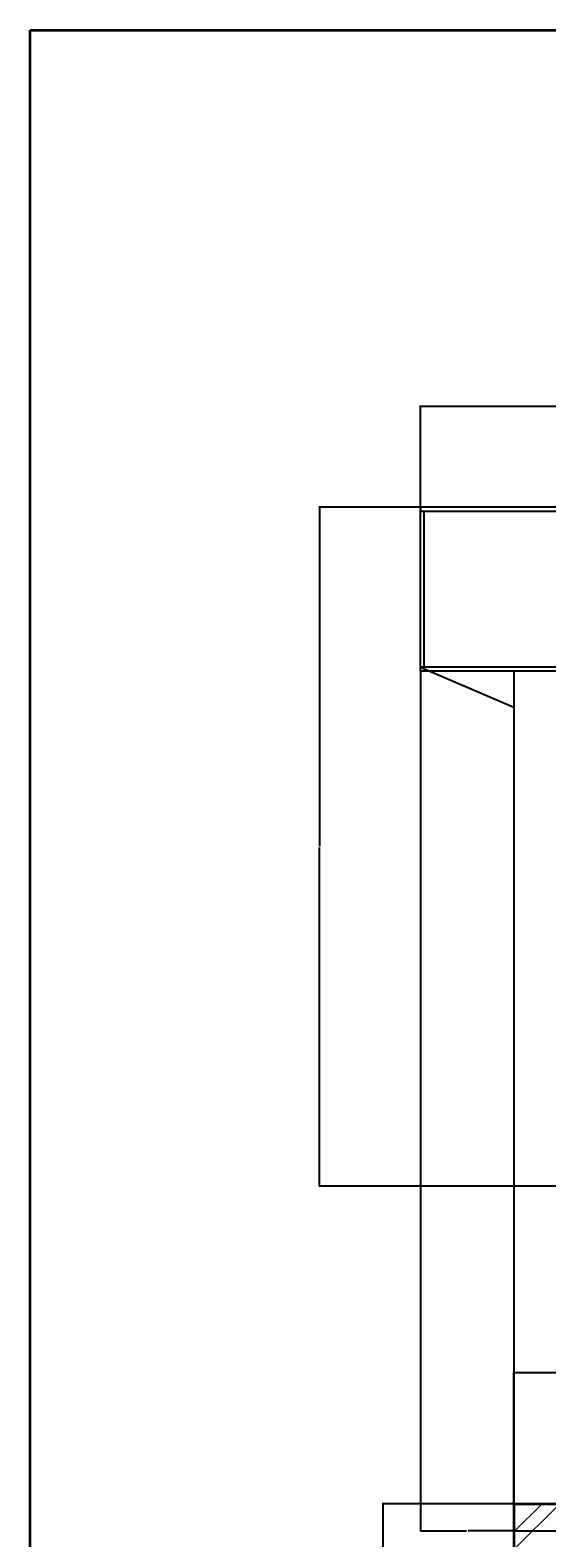
# Model space of a CAD drawing. Units: inches. Extents: x 1152 to 2588, y 1459 to 2618.
# Tile 7 of 17: x 1152 to 1285, y 2231 to 2618. Entities that reach past the tile are written whole.
import ezdxf

# ---------------------------------------------------------------- set-up
doc = ezdxf.new("R2010")
doc.units = ezdxf.units.IN
for name, color, linetype, lineweight in [('A-ANNO-DIMS', 2, 'Continuous', 18), ('A-ANNO-TTLB', 7, 'Continuous', 35), ('A-ELEV', 7, 'Continuous', 25), ('A-WALL', 7, 'Continuous', 35), ('A-WALL-PATT', 8, 'Continuous', 13)]:
    doc.layers.add(name, color=color, linetype=linetype, lineweight=lineweight)
doc.styles.get("Standard").update_dxf_attribs({"font": 'arial.ttf'})
doc.dimstyles.get("Standard").update_dxf_attribs({"dimtxt": 0.18, "dimasz": 0.18, "dimexe": 0.18, "dimexo": 0.0625, "dimgap": 0.09, "dimtad": 0, "dimtih": 1, "dimtoh": 1, "dimdec": 4, "dimzin": 0, "dimdsep": 46, "dimtxsty": 'Standard', "dimcen": 0.09, "dimadec": 0, "dimazin": 0, "dimtfac": 1, "dimtdec": 4, "dimtofl": 0, "dimtmove": 0, "dimatfit": 3, "dimfxl": 1, "dimtolj": 1, "dimtzin": 0, "dimarcsym": 0})

# ---------------------------------------------------------------- blocks, each defined once
blk = doc.blocks.new('*D70')
at = {"layer": 'A-ANNO-DIMS', "color": 0, "lineweight": -2, "transparency": 16777216}
for p, q in [((1276.42, 2240.11), (1276.42, 2273.83)), ((1276.6, 2273.65), (1506.12, 2273.65)), ((1736.24, 2273.65), (1506.71, 2273.65)), ((1736.42, 2240.11), (1736.42, 2273.83))]:
    blk.add_line(p, q, dxfattribs=at)
at = {"layer": 'A-ANNO-DIMS', "color": 0, "transparency": 16777216}
for points in [[(1276.6, 2273.68), (1276.6, 2273.62), (1276.42, 2273.65)], [(1736.24, 2273.68), (1736.24, 2273.62), (1736.42, 2273.65)]]:
    blk.add_solid(points, dxfattribs=at)
at = {"layer": 'Defpoints', "color": 0, "transparency": 16777216}
for p in [(1736.42, 2273.65), (1276.42, 2240.05), (1736.42, 2240.05)]:
    blk.add_point(p, dxfattribs=at)
at = {"layer": 'A-ANNO-DIMS', "color": 0, "transparency": 16777216, "insert": (1506.42, 2273.65), "char_height": 0.18, "attachment_point": 5}
blk.add_mtext('\\A1;460', dxfattribs=at)
blk = doc.blocks.new('*D71')
at = {"layer": 'A-ANNO-DIMS', "color": 0, "lineweight": -2, "transparency": 16777216}
for p, q in [((1276.35, 2240.05), (1242.64, 2240.05)), ((1242.82, 2239.87), (1242.82, 1937.73)), ((1242.82, 1635.23), (1242.82, 1937.36)), ((1276.35, 1635.05), (1242.64, 1635.05))]:
    blk.add_line(p, q, dxfattribs=at)
at = {"layer": 'A-ANNO-DIMS', "color": 0, "transparency": 16777216}
for points in [[(1242.79, 2239.87), (1242.85, 2239.87), (1242.82, 2240.05)], [(1242.79, 1635.23), (1242.85, 1635.23), (1242.82, 1635.05)]]:
    blk.add_solid(points, dxfattribs=at)
at = {"layer": 'Defpoints', "color": 0, "transparency": 16777216}
for p in [(1242.82, 2240.05), (1276.42, 2240.05), (1276.42, 1635.05)]:
    blk.add_point(p, dxfattribs=at)
at = {"layer": 'A-ANNO-DIMS', "color": 0, "transparency": 16777216, "insert": (1242.82, 1937.55), "char_height": 0.18, "attachment_point": 5}
blk.add_mtext('\\A1;605', dxfattribs=at)
blk = doc.blocks.new('*D88')
at = {"layer": 'A-ANNO-DIMS', "color": 0, "lineweight": -2, "transparency": 16777216}
for p, q in [((1252.42, 2495.45), (1252.42, 2521.47)), ((1252.6, 2521.29), (1506.13, 2521.29)), ((1760.24, 2521.29), (1506.71, 2521.29)), ((1760.42, 2495.45), (1760.42, 2521.47))]:
    blk.add_line(p, q, dxfattribs=at)
at = {"layer": 'A-ANNO-DIMS', "color": 0, "transparency": 16777216}
for points in [[(1252.6, 2521.32), (1252.6, 2521.26), (1252.42, 2521.29)], [(1760.24, 2521.32), (1760.24, 2521.26), (1760.42, 2521.29)]]:
    blk.add_solid(points, dxfattribs=at)
at = {"layer": 'Defpoints', "color": 0, "transparency": 16777216}
for p in [(1760.42, 2521.29), (1252.42, 2495.39), (1760.42, 2495.39)]:
    blk.add_point(p, dxfattribs=at)
at = {"layer": 'A-ANNO-DIMS', "color": 0, "transparency": 16777216, "insert": (1506.42, 2521.29), "char_height": 0.18, "attachment_point": 5}
blk.add_mtext('\\A1;508', dxfattribs=at)
blk = doc.blocks.new('*D89')
at = {"layer": 'A-ANNO-DIMS', "color": 0, "lineweight": -2, "transparency": 16777216}
for p, q in [((1252.35, 2495.39), (1226.34, 2495.39)), ((1226.52, 2495.21), (1226.52, 2408.57)), ((1226.52, 2321.57), (1226.52, 2408.21)), ((1276.35, 2321.39), (1226.34, 2321.39))]:
    blk.add_line(p, q, dxfattribs=at)
at = {"layer": 'A-ANNO-DIMS', "color": 0, "transparency": 16777216}
for points in [[(1226.49, 2495.21), (1226.55, 2495.21), (1226.52, 2495.39)], [(1226.49, 2321.57), (1226.55, 2321.57), (1226.52, 2321.39)]]:
    blk.add_solid(points, dxfattribs=at)
at = {"layer": 'Defpoints', "color": 0, "transparency": 16777216}
for p in [(1226.52, 2495.39), (1252.42, 2495.39), (1276.42, 2321.39)]:
    blk.add_point(p, dxfattribs=at)
at = {"layer": 'A-ANNO-DIMS', "color": 0, "transparency": 16777216, "insert": (1226.52, 2408.39), "char_height": 0.18, "attachment_point": 5}
blk.add_mtext('\\A1;174', dxfattribs=at)
blk = doc.blocks.new('*D90')
at = {"layer": 'A-ANNO-DIMS', "color": 0, "lineweight": -2, "transparency": 16777216}
for p, q in [((1252.42, 2453.33), (1252.42, 2232.94)), ((1276.42, 2321.33), (1276.42, 2232.94)), ((1252.6, 2233.12), (1264.2, 2233.12)), ((1276.24, 2233.12), (1264.64, 2233.12))]:
    blk.add_line(p, q, dxfattribs=at)
at = {"layer": 'A-ANNO-DIMS', "color": 0, "transparency": 16777216}
for points in [[(1252.6, 2233.15), (1252.6, 2233.09), (1252.42, 2233.12)], [(1276.24, 2233.15), (1276.24, 2233.09), (1276.42, 2233.12)]]:
    blk.add_solid(points, dxfattribs=at)
at = {"layer": 'Defpoints', "color": 0, "transparency": 16777216}
for p in [(1252.42, 2453.39), (1276.42, 2321.39), (1276.42, 2233.12)]:
    blk.add_point(p, dxfattribs=at)
at = {"layer": 'A-ANNO-DIMS', "color": 0, "transparency": 16777216, "insert": (1264.42, 2233.12), "char_height": 0.18, "attachment_point": 5}
blk.add_mtext('\\A1;24', dxfattribs=at)
blk = doc.blocks.new('*D91')
at = {"layer": 'A-ANNO-DIMS', "color": 0, "lineweight": -2, "transparency": 16777216}
for p, q in [((1405.42, 2327.33), (1405.42, 2232.94)), ((1276.42, 2321.33), (1276.42, 2232.94)), ((1276.6, 2233.12), (1340.64, 2233.12)), ((1405.24, 2233.12), (1341.2, 2233.12))]:
    blk.add_line(p, q, dxfattribs=at)
at = {"layer": 'A-ANNO-DIMS', "color": 0, "transparency": 16777216}
for points in [[(1276.6, 2233.15), (1276.6, 2233.09), (1276.42, 2233.12)], [(1405.24, 2233.15), (1405.24, 2233.09), (1405.42, 2233.12)]]:
    blk.add_solid(points, dxfattribs=at)
at = {"layer": 'Defpoints', "color": 0, "transparency": 16777216}
for p in [(1405.42, 2327.39), (1276.42, 2321.39), (1405.42, 2233.12)]:
    blk.add_point(p, dxfattribs=at)
at = {"layer": 'A-ANNO-DIMS', "color": 0, "transparency": 16777216, "insert": (1340.92, 2233.12), "char_height": 0.18, "attachment_point": 5}
blk.add_mtext('\\A1;129', dxfattribs=at)

msp = doc.modelspace()

# ---------------------------------------------------------------- hatches: boundary and pattern name
at = {"layer": 'A-WALL-PATT'}
h = msp.add_hatch(dxfattribs=at)
h.set_pattern_fill('ANSI32', color=256)
h.paths.add_polyline_path([(1408.9272, 2240.0458), (1276.4165, 2240.0458), (1276.4165, 2192.7491), (1285.4165, 2192.7491), (1285.4165, 2231.0458), (1369.4165, 2231.0458), (1369.4165, 2084.0458), (1526.9165, 2084.0458), (1526.9165, 2096.3728), (1524.6665, 2096.3728), (1522.4165, 2096.3728), (1522.4165, 2093.0458), (1378.4165, 2093.0458), (1378.4165, 2231.0458), (1408.9272, 2231.0458)])
h.paths.add_polyline_path([(1736.4165, 2240.0458), (1468.9272, 2240.0458), (1468.9272, 2231.0458), (1522.4165, 2231.0458), (1522.4165, 2127.3313), (1526.9165, 2127.3313), (1526.9165, 2231.0458), (1574.9165, 2231.0458), (1574.9165, 2188.0458), (1579.4165, 2188.0458), (1579.4165, 2231.0458), (1727.4165, 2231.0458), (1727.4165, 2183.9728), (1736.4165, 2183.9728)])
h.paths.add_polyline_path([(1285.4165, 2156.7491), (1276.4165, 2156.7491), (1276.4165, 2084.0458), (1285.4165, 2084.0458)], flags=17)
h.paths.add_polyline_path([(1285.4165, 2043.5458), (1445.4165, 2043.5458), (1445.4165, 1943.6503), (1454.4165, 1943.6503), (1454.4165, 2048.0458), (1276.4165, 2048.0458), (1276.4165, 2019.2077), (1280.9165, 2019.2077), (1285.4165, 2019.2077)])
h.paths.add_polyline_path([(1285.4165, 1959.2077), (1276.4165, 1959.2077), (1276.4165, 1891.1319), (1280.9165, 1891.1319), (1285.4165, 1891.1319), (1285.4165, 1901.0458), (1376.8505, 1901.0458), (1376.8505, 1903.2958), (1376.8505, 1905.5458), (1285.4165, 1905.5458)])
h.paths.add_polyline_path([(1518.4165, 1905.5458), (1399.2832, 1905.5458), (1399.2832, 1903.2958), (1399.2832, 1901.0458), (1405.4165, 1901.0458), (1405.4165, 1884.8579), (1409.9165, 1884.8579), (1409.9165, 1901.0458), (1513.9165, 1901.0458), (1513.9165, 1869.1706), (1518.4165, 1869.1706)])
h.paths.add_polyline_path([(1520.5229, 1845.0458), (1518.4165, 1845.0458), (1518.4165, 1849.2927), (1516.1665, 1849.2927), (1513.9165, 1849.2927), (1513.9165, 1845.0458), (1409.9165, 1845.0458), (1409.9165, 1860.8579), (1405.4165, 1860.8579), (1405.4165, 1845.0458), (1285.4165, 1845.0458), (1285.4165, 1867.1319), (1276.4165, 1867.1319), (1276.4165, 1635.0458), (1285.4165, 1635.0458), (1285.4165, 1836.0458), (1405.4165, 1836.0458), (1405.4165, 1635.0458), (1414.4165, 1635.0458), (1424.7277, 1635.0458), (1424.7277, 1639.5458), (1424.7277, 1644.0458), (1414.4165, 1644.0458), (1414.4165, 1836.0458), (1414.4165, 1840.5831), (1520.5229, 1840.5831)])
h.paths.add_polyline_path([(1579.4165, 1840.5458), (1583.4035, 1840.5458), (1583.4035, 1845.0458), (1579.4165, 1845.0458), (1570.4165, 1845.0458), (1570.4165, 1840.5831), (1570.4165, 1644.0458), (1548.2359, 1644.0458), (1548.2359, 1635.0458), (1611.2801, 1635.0458), (1611.2801, 1639.5458), (1611.2801, 1644.0458), (1579.4165, 1644.0458)])
h.paths.add_polyline_path([(1488.2359, 1644.0458), (1472.0663, 1644.0458), (1472.0663, 1635.0458), (1488.2359, 1635.0458), (1488.2359, 1639.5458)], flags=17)
h.paths.add_polyline_path([(1736.4165, 1701.1863), (1727.4165, 1701.1863), (1727.4165, 1644.0458), (1671.2801, 1644.0458), (1671.2801, 1635.0458), (1736.4165, 1635.0458)])
h.paths.add_polyline_path([(1736.4165, 2147.9728), (1727.4165, 2147.9728), (1727.4165, 2093.0458), (1579.4165, 2093.0458), (1574.9165, 2093.0458), (1574.9165, 1971.6501), (1579.4165, 1971.6501), (1579.4165, 2084.0458), (1727.4165, 2084.0458), (1727.4165, 2054.3847), (1736.4165, 2054.3847)])
h.paths.add_polyline_path([(1736.4165, 1994.3847), (1727.4165, 1994.3847), (1727.4165, 1911.3562), (1736.4165, 1911.3562)])
h.paths.add_polyline_path([(1736.4165, 1875.3562), (1727.4165, 1875.3562), (1727.4165, 1845.0458), (1617.1767, 1845.0458), (1617.1767, 1842.7958), (1617.1767, 1840.5458), (1618.9165, 1840.5458), (1618.9165, 1788.5458), (1618.9165, 1784.0458), (1627.8699, 1784.0458), (1627.8699, 1788.5458), (1623.4165, 1788.5458), (1623.4165, 1840.5458), (1727.4165, 1840.5458), (1727.4165, 1828.7619), (1736.4165, 1828.7619)])
h.paths.add_polyline_path([(1727.4165, 1938.0458), (1579.4165, 1938.0458), (1579.4165, 1942.7722), (1574.9165, 1942.7722), (1574.9165, 1929.0458), (1727.4165, 1929.0458)])

# ---------------------------------------------------------------- linework, layer by layer
at = {"layer": 'A-ANNO-TTLB'}
msp.add_lwpolyline([(1152.3215, 2617.6685), (2587.6987, 2617.6685), (2587.6987, 1459.3148), (1152.3215, 1459.3148)], close=True, dxfattribs=at)
at = {"layer": 'A-ELEV'}
for p, q in [((1760.4165, 2495.3911), (1252.4165, 2495.3911)), ((1252.4165, 2453.3911), (1252.4165, 2495.3911)), ((1252.4165, 2495.3911), (1252.4165, 2494.3911)), ((1252.4165, 2494.3911), (1760.4165, 2494.3911)), ((1253.4165, 2454.3911), (1253.4165, 2494.3911)), ((1759.4165, 2454.3911), (1252.4165, 2454.3911)), ((1252.4165, 2454.3911), (1253.4165, 2454.3911)), ((1252.4165, 2454.3911), (1276.4165, 2444.1872)), ((1760.4165, 2453.3911), (1252.4165, 2453.3911)), ((1276.4165, 2453.3911), (1276.4165, 2321.3911)), ((1736.4165, 2321.3911), (1276.4165, 2321.3911))]:
    msp.add_line(p, q, dxfattribs=at)
at = {"layer": 'A-WALL'}
for q in [(1736.4165, 2240.0458), (1276.4165, 2084.0458)]:
    msp.add_line((1276.4165, 2240.0458), q, dxfattribs=at)

# ---------------------------------------------------------------- dimensions: what is measured, and where the dimension line sits
at = {"layer": 'A-ANNO-DIMS'}
for base, p1, p2, picture, middle in [((1760.4165, 2521.2911), (1252.4165, 2495.3911), (1760.4165, 2495.3911), '*D88', (1506.4165, 2521.2911)), ((1276.4165, 2233.12), (1252.4165, 2453.3911), (1276.4165, 2321.3911), '*D90', (1264.4165, 2233.12)), ((1405.4165, 2233.12), (1276.4165, 2321.3911), (1405.4165, 2327.3911), '*D91', (1340.9165, 2233.12)), ((1736.4165, 2273.6458), (1276.4165, 2240.0458), (1736.4165, 2240.0458), '*D70', (1506.4165, 2273.6458))]:
    dim = msp.add_linear_dim(base=base, p1=p1, p2=p2, dimstyle='Standard', override={"dimdec": 0, "dimlfac": 1, "dimrnd": 0, "dimzin": 0, "dimdsep": 46, "dimlunit": 2}, dxfattribs=at)
    dim.commit()
    dim.dimension.update_dxf_attribs({"geometry": picture, "text_midpoint": middle})
for base, p1, p2, picture, middle in [((1226.5165, 2495.3911), (1276.4165, 2321.3911), (1252.4165, 2495.3911), '*D89', (1226.5165, 2408.3911)), ((1242.8165, 2240.0458), (1276.4165, 1635.0458), (1276.4165, 2240.0458), '*D71', (1242.8165, 1937.5458))]:
    dim = msp.add_linear_dim(base=base, p1=p1, p2=p2, angle=90, dimstyle='Standard', override={"dimdec": 0, "dimlfac": 1, "dimrnd": 0, "dimzin": 0, "dimdsep": 46, "dimlunit": 2}, dxfattribs=at)
    dim.commit()
    dim.dimension.update_dxf_attribs({"geometry": picture, "text_midpoint": middle})

doc.saveas('drawing.dxf')
